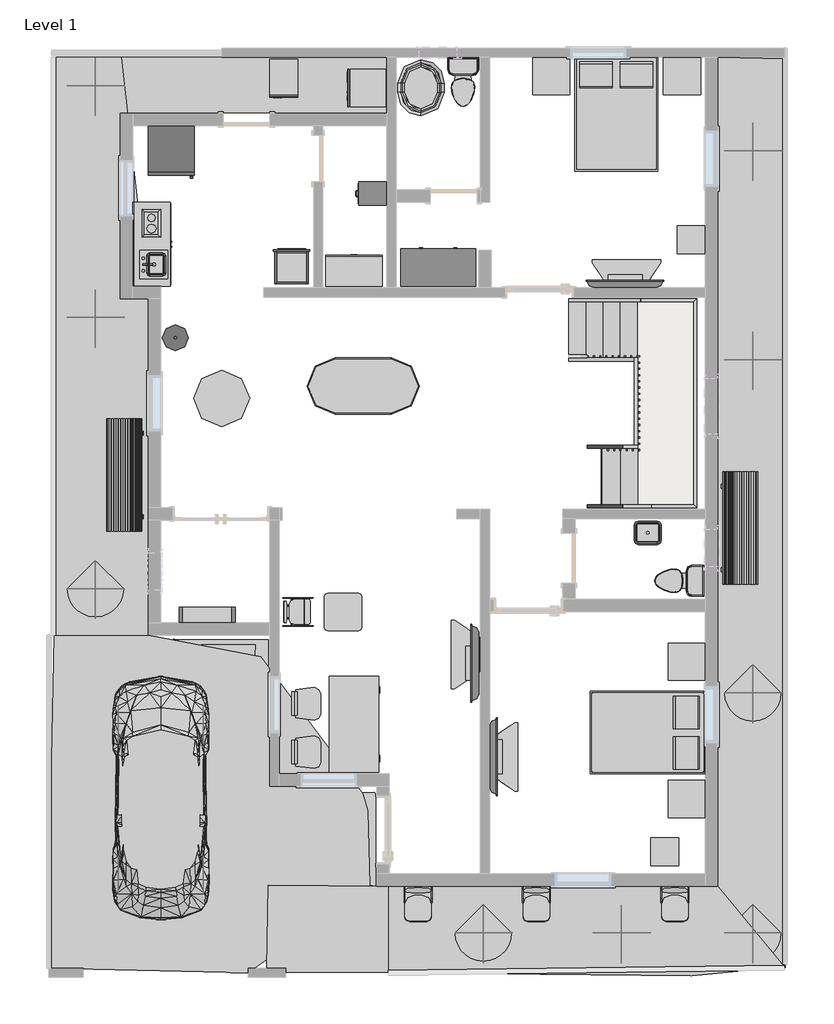
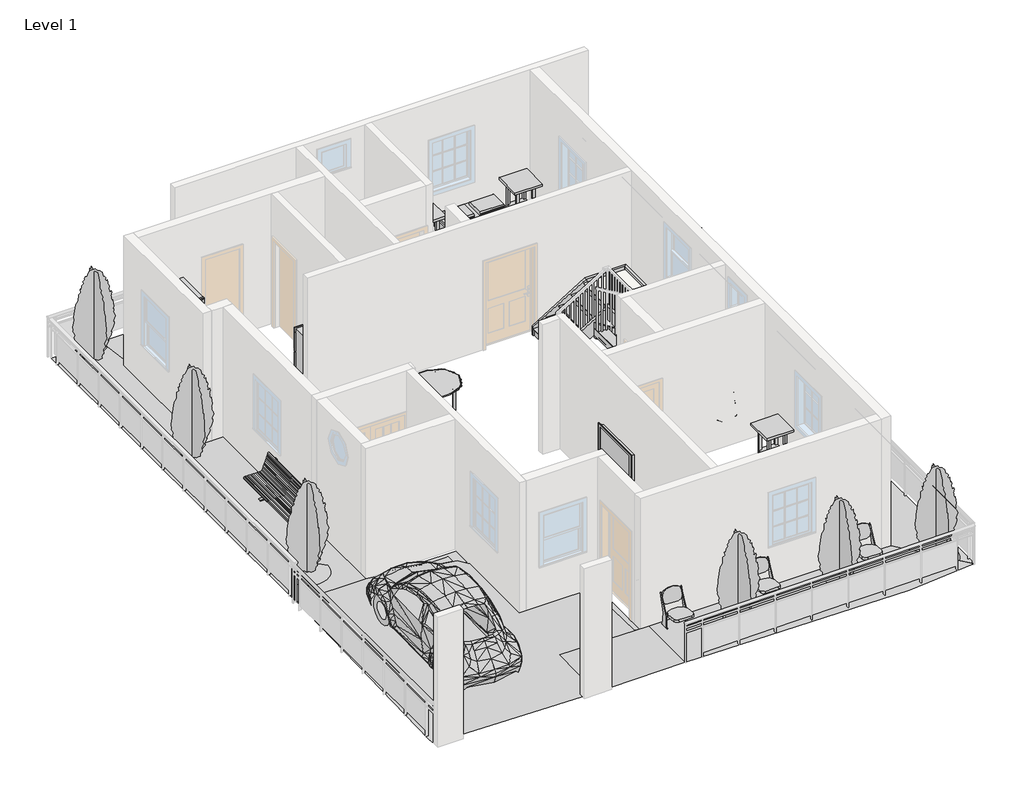
# One storey, part 4 of 4: 29 furniture elements, 16 proxies, 11 geographic elements, 8 members, 6 flow terminals, 2 stair flights, 1 slab.
"""IFC4 building model written with IfcOpenShell, lengths in millimetres."""

from ifc_helpers import new_model, si_unit, frame, origin, place, context, project, spatial, polyline, outline, extrude, faceted_brep, triangles, transform, mapped, element, save
from components import proxy_7e1014cc, proxy_fe84b772, proxy_45b28599, proxy_844211aa, proxy_8b8c2dc4, rpc_beetle_rpc_beetle_3ce7ba48, proxy_a13a33b2, flow_terminal_871c2e40, flow_terminal_d49f872f, flow_terminal_62a433f7, toilet_domestic_3d_toilet_domestic_3d_f7549cf7, toilet_domestic_3d_toilet_domestic_3d_183bbd19, flow_terminal_2ca5ee5d, furniture_c8abb964, furniture_b1353b55, chair_desk_chair_desk_ccc35c8f, chair_stacking_chair_stacking_4df0970f, furniture_95afb093, furniture_013ab306, furniture_9fa109b2, furniture_3d1d9cbc, furniture_417d203a, furniture_e1dba61b, furniture_fdf74506, tv_stand_tv_stand_6ce107e5, furniture_2c34a4f9, furniture_905aceb5, furniture_bcf351fa, furniture_097b63cf, furniture_5bc9ed15, geographic_element_235d1464, rpc_tree_conifer_chinese_juniper_7_1b9786cd, non_monolithic_landing_bdf883c6, stair_flight_1d7161dd, stair_flight_6800fc22

model = new_model("IFC4")

# Units and contexts
model_context = context("Model", 3, world=origin())
ifc_project = project(units=[si_unit("LENGTHUNIT", "METRE", prefix="MILLI")], contexts=[model_context])

# Site, building, storey
site = spatial("IfcSite", under=ifc_project)
building = spatial("IfcBuilding", under=site)
storey = spatial("IfcBuildingStorey", under=building, Name="Level 1", Elevation=0.0)

# Proxies
placement = place(None, origin())
element("IfcBuildingElementProxy", 1, Name="Building Element Proxy", at=placement, inside=storey, context=model_context, shape_type="Tessellation", body=[
    triangles([(-6292.1432602, 15373.2430298, 0.0), (-5213.9224457, 15356.2475555, 0.0), (-6292.1432602, 1860.4426907, 0.0), (-5190.4186478, 530.1176785, 0.0)], [[1, 3, 2], [4, 2, 3]], closed=False),
])
element("IfcBuildingElementProxy", 2, Name="Building Element Proxy", at=placement, inside=storey, context=model_context, shape_type="Tessellation", body=[
    triangles([(-6292.1432602, 1860.4426907, 0.0), (-5209.4686478, 549.1676785, 0.0), (-6721.6182083, 398.6723588, 0.0), (-11662.7439331, 449.442661, 0.0), (-11662.7439331, 1860.4426907, 0.0)], [[5, 4, 3], [3, 2, 1], [3, 1, 5]], closed=False),
])
element("IfcBuildingElementProxy", 3, Name="Building Element Proxy", at=placement, inside=storey, context=model_context, shape_type="Tessellation", body=[
    triangles([(-13339.1439331, 449.442661, 0.0), (-11669.2121429, 458.8875423, 0.0), (-11662.7439331, 1860.4426907, 0.0), (-13622.0394562, 1880.1632893, 0.0), (-13643.9439331, 525.642661, 0.0)], [[4, 5, 1], [1, 2, 3], [1, 3, 4]], closed=False),
])
element("IfcBuildingElementProxy", 4, Name="Building Element Proxy", at=placement, inside=storey, context=model_context, shape_type="Tessellation", body=[
    triangles([(-15577.8398438, 5952.1611053, 0.0), (-17123.743158, 5952.1611053, 0.0), (-15577.8398438, 11438.5611053, 0.0), (-16035.0398438, 11438.5611053, 0.0), (-16021.9080872, 15373.2430298, 0.0), (-17123.743158, 15373.2430298, 0.0)], [[6, 2, 4], [4, 2, 1], [6, 4, 5], [4, 3, 5], [3, 4, 1]], closed=False),
])
element("IfcBuildingElementProxy", 5, Name="Building Element Proxy", at=placement, inside=storey, context=model_context, shape_type="Tessellation", body=[
    triangles([(-16013.146994, 15373.2430298, 0.0), (-16019.2815033, 15373.2430298, 0.0), (-15917.9969879, 14469.5377258, 0.0), (-11691.6398438, 14461.1614929, 0.0), (-11691.6398438, 15373.2430298, 0.0)], [[3, 5, 1], [1, 2, 3], [3, 4, 5]], closed=False),
])
element("IfcBuildingElementProxy", 6, Name="Building Element Proxy", at=placement, inside=storey, context=model_context, shape_type="Tessellation", body=[
    triangles([(-17114.218158, 5945.8109116, 0.0), (-15577.8398438, 5952.1611053, 0.0), (-15719.3253937, 5575.8137283, 0.0), (-13765.4318665, 5526.4318588, 0.0), (-13747.9236328, 5599.4901901, 0.0), (-13732.6571228, 3093.6073906, 0.0), (-11998.7943512, 3091.0264435, 0.0), (-11972.09133, 1876.438662, 0.0), (-13622.0394562, 1891.7326412, 0.0), (-16641.1435455, 525.642661, 0.0), (-17217.7350952, 675.719874, 0.0), (-17199.943158, 525.642661, 0.0), (-13948.7439331, 449.442661, 0.0), (-12085.333255, 3366.7753098, 0.0)], [[12, 13, 10], [6, 11, 10], [12, 10, 11], [1, 11, 3], [3, 2, 1], [6, 3, 11], [3, 4, 2], [9, 10, 13], [9, 8, 7], [8, 9, 13], [9, 7, 6], [4, 5, 2], [5, 4, 14], [6, 14, 4], [14, 6, 7], [4, 3, 6], [9, 6, 10]], closed=False),
])
element("IfcBuildingElementProxy", 7, Name="Building Element Proxy", at=placement, inside=storey, context=model_context, shape_type="Tessellation", body=[
    triangles([(-13839.5657135, 5779.0495789, 0.0), (-13853.3788239, 5648.8115982, 0.0), (-14738.6096741, 5792.6731659, 0.0), (-13837.1100494, 5794.7480392, 0.0), (-13844.1212494, 5616.9437759, 0.0), (-14719.3480591, 5791.5819534, 0.0), (-14720.0968506, 5784.5259888, 0.0)], [[3, 7, 6], [6, 7, 2], [3, 6, 4], [2, 5, 1], [5, 2, 7], [1, 4, 6], [4, 1, 5], [2, 1, 6]], closed=False),
])
element("IfcBuildingElementProxy", 8, Name="Building Element Proxy", at=placement, inside=storey, context=model_context, shape_type="Tessellation", body=[
    triangles([(-11869.4394562, 3361.3611053, 0.0), (-11892.5240936, 3389.4227646, 0.0), (-12081.1823456, 3388.4777641, 0.0), (-11869.4394562, 1862.7610085, 0.0), (-11970.361203, 1873.1361019, 0.0), (-12092.2537628, 3386.2162743, 0.0)], [[3, 6, 1], [1, 6, 5], [3, 1, 2], [1, 5, 4]], closed=False),
])
element("IfcBuildingElementProxy", 9, Name="Building Element Proxy", at=placement, inside=storey, context=model_context, shape_type="Tessellation", body=[
    triangles([(-13622.0394562, 5455.0077301, 0.0), (-13622.0394562, 5882.7031357, 0.0), (-15168.4729706, 5887.4801697, 0.0)], [[3, 1, 2]], closed=False),
])
proxy_shape = proxy_7e1014cc(model_context)
element("IfcBuildingElementProxy", 10, Name="18\" x 24\" x 34 1/2\"", ObjectType="18\" x 24\" x 34 1/2\"", at=placement, inside=storey, context=model_context, shape_type="MappedRepresentation", body=[
    mapped(proxy_shape, transform((-13674.1574653, 14776.5930991, 0.0), x_axis=(1.0, 0.0, 0.0), y_axis=(0.0, 1.0, 0.0), z_axis=(0.0, 0.0, 1.0))),
])
proxy_2_shape = proxy_fe84b772(model_context)
element("IfcBuildingElementProxy", 11, Name="Cook Top-2 Unit : 12\" x 18\"", ObjectType="Cook Top-2 Unit : 12\" x 18\"", at=placement, inside=storey, context=model_context, shape_type="MappedRepresentation", body=[
    mapped(proxy_2_shape, transform((-15450.8399968, 12700.6858539, 0.0), x_axis=(-1.0, 0.0, 0.0), y_axis=(0.0, -1.0, 0.0), z_axis=(0.0, 0.0, 1.0))),
])
proxy_3_shape = proxy_45b28599(model_context)
element("IfcBuildingElementProxy", 12, Name="Dishwasher : 24\" x 24\" x 34\"", ObjectType="Dishwasher : 24\" x 24\" x 34\"", at=placement, inside=storey, context=model_context, shape_type="MappedRepresentation", body=[
    mapped(proxy_3_shape, transform((-12277.1574653, 15259.1930991, 0.0), x_axis=(0.0, -1.0000000000000007, 0.0), y_axis=(1.0000000000000007, 0.0, 0.0), z_axis=(0.0, 0.0, 1.0))),
])
proxy_4_shape = proxy_844211aa(model_context)
element("IfcBuildingElementProxy", 13, Name="Kitchenette - Small : 54\"", ObjectType="Kitchenette - Small : 54\"", at=placement, inside=storey, context=model_context, shape_type="MappedRepresentation", body=[
    mapped(proxy_4_shape, transform((-15831.8399968, 12308.8233534, 0.0), x_axis=(0.0, 1.0, 0.0), y_axis=(-1.0, 0.0, 0.0), z_axis=(0.0, 0.0, 1.0))),
])
proxy_5_shape = proxy_8b8c2dc4(model_context)
element("IfcBuildingElementProxy", 14, Name="Oven Double-Built-in : 21 1/2\" x 39 1/4\" x 21\"", ObjectType="Oven Double-Built-in : 21 1/2\" x 39 1/4\" x 21\"", at=placement, inside=storey, context=model_context, shape_type="MappedRepresentation", body=[
    mapped(proxy_5_shape, transform((-13276.2149241, 12087.6269172, 0.0), x_axis=(-1.0000000000000004, 0.0, 0.0), y_axis=(0.0, -1.0000000000000004, 0.0), z_axis=(0.0, 0.0, 1.0))),
])
rpc_beetle_rpc_beetle_shape = rpc_beetle_rpc_beetle_3ce7ba48(model_context)
element("IfcBuildingElementProxy", 15, Name="RPC Beetle : RPC Beetle", ObjectType="RPC Beetle : RPC Beetle", at=placement, inside=storey, context=model_context, shape_type="MappedRepresentation", body=[
    mapped(rpc_beetle_rpc_beetle_shape, transform((-15374.6399968, 2063.6426639, 0.0), x_axis=(1.0, 0.0, 0.0), y_axis=(0.0, 1.0, 0.0), z_axis=(0.0, 0.0, 1.0))),
])
proxy_6_shape = proxy_a13a33b2(model_context)
element("IfcBuildingElementProxy", 16, Name="Refrigerator : 30\" x 32\" RH", ObjectType="Refrigerator : 30\" x 32\" RH", at=placement, inside=storey, context=model_context, shape_type="MappedRepresentation", body=[
    mapped(proxy_6_shape, transform((-15204.7774968, 13869.4120868, 0.0), x_axis=(1.0, 0.0, 0.0), y_axis=(0.0, 1.0, 0.0), z_axis=(0.0, 0.0, 1.0))),
])

# Flow terminals
flow_terminal_shape = flow_terminal_871c2e40(model_context)
element("IfcFlowTerminal", 17, ObjectType="Sink Kitchen-Island : 18\" x 18\"", at=placement, inside=storey, context=model_context, shape_type="MappedRepresentation", body=[
    mapped(flow_terminal_shape, transform((-15486.5945957, 11981.6718177, 0.0), x_axis=(0.0, 1.0, 0.0), y_axis=(-1.0, 0.0, 0.0), z_axis=(0.0, 0.0, 1.0))),
])
flow_terminal_2_shape = flow_terminal_d49f872f(model_context)
element("IfcFlowTerminal", 18, ObjectType="Sink Vanity-Round : 19\" x 19\"", at=placement, inside=storey, context=model_context, shape_type="MappedRepresentation", body=[
    mapped(flow_terminal_2_shape, transform((-15053.3054094, 10706.9093177, 609.6), x_axis=(0.0, 1.0000000000000002, 0.0), y_axis=(-1.0000000000000002, 0.0, 0.0), z_axis=(0.0, 0.0, 1.0))),
])
flow_terminal_3_shape = flow_terminal_62a433f7(model_context)
element("IfcFlowTerminal", 19, ObjectType="Sink Vanity-Square : 20\" x 18\"", at=placement, inside=storey, context=model_context, shape_type="MappedRepresentation", body=[
    mapped(flow_terminal_3_shape, transform((-7450.8327199, 7674.6972628, 609.6), x_axis=(1.0, 0.0, 0.0), y_axis=(0.0, 1.0, 0.0), z_axis=(0.0, 0.0, 1.0))),
])
toilet_domestic_3d_toilet_domestic_3d_shape = toilet_domestic_3d_toilet_domestic_3d_f7549cf7(model_context)
toilet_domestic_3d_toilet_domestic_3d_2_shape = toilet_domestic_3d_toilet_domestic_3d_183bbd19(model_context)
element("IfcFlowTerminal", 20, ObjectType="Toilet-Domestic-3D : Toilet-Domestic-3D", at=placement, inside=storey, context=model_context, shape_type="MappedRepresentation", body=[
    mapped(toilet_domestic_3d_toilet_domestic_3d_shape, transform((-7015.4395067, 6841.1610583, 0.0), x_axis=(0.0, -1.0000000000000002, 0.0), y_axis=(1.0000000000000002, 0.0, 0.0), z_axis=(0.0, 0.0, 1.0))),
    mapped(toilet_domestic_3d_toilet_domestic_3d_2_shape, transform((-7015.4395067, 6841.1610583, 0.0), x_axis=(0.0, -1.0000000000000002, 0.0), y_axis=(1.0000000000000002, 0.0, 0.0), z_axis=(0.0, 0.0, 1.0))),
])
element("IfcFlowTerminal", 21, ObjectType="Toilet-Domestic-3D : Toilet-Domestic-3D", at=placement, inside=storey, context=model_context, shape_type="MappedRepresentation", body=[
    mapped(toilet_domestic_3d_toilet_domestic_3d_shape, transform((-10447.0399968, 14878.5466366, 0.0), x_axis=(1.0, 0.0, 0.0), y_axis=(0.0, 1.0, 0.0), z_axis=(0.0, 0.0, 1.0))),
    mapped(toilet_domestic_3d_toilet_domestic_3d_2_shape, transform((-10447.0399968, 14878.5466366, 0.0), x_axis=(1.0, 0.0, 0.0), y_axis=(0.0, 1.0, 0.0), z_axis=(0.0, 0.0, 1.0))),
])
flow_terminal_4_shape = flow_terminal_2ca5ee5d(model_context)
element("IfcFlowTerminal", 22, ObjectType="Tub-Free Standing-3D : 30\" x 60\"", at=placement, inside=storey, context=model_context, shape_type="MappedRepresentation", body=[
    mapped(flow_terminal_4_shape, transform((-11132.8399968, 14878.5466366, 0.0), x_axis=(1.0, 0.0, 0.0), y_axis=(0.0, 1.0, 0.0), z_axis=(0.0, 0.0, 1.0))),
])

# Furniture
furniture_shape = furniture_c8abb964(model_context)
element("IfcFurniture", 23, ObjectType="Bed-Box : Double 53\" x 74\"", at=placement, inside=storey, context=model_context, shape_type="MappedRepresentation", body=[
    mapped(furniture_shape, transform((-8288.0399968, 14695.5905665, 0.0), x_axis=(1.0, 0.0, 0.0), y_axis=(0.0, 1.0, 0.0), z_axis=(0.0, 0.0, 1.0))),
])
element("IfcFurniture", 24, ObjectType="Bed-Box : Double 53\" x 74\"", at=placement, inside=storey, context=model_context, shape_type="MappedRepresentation", body=[
    mapped(furniture_shape, transform((-7200.7139711, 4703.8135173, 0.0), x_axis=(0.0, -0.9999999999999999, 0.0), y_axis=(0.9999999999999999, 0.0, 0.0), z_axis=(0.0, 0.0, 1.0))),
])
furniture_2_shape = furniture_b1353b55(model_context)
element("IfcFurniture", 25, ObjectType="Cabinet-File 4 Drawer : 15\" x 18\"", at=placement, inside=storey, context=model_context, shape_type="MappedRepresentation", body=[
    mapped(furniture_2_shape, transform((-11778.1056967, 13025.1646112, 0.0), x_axis=(0.0, -0.9999999999999998, 0.0), y_axis=(0.9999999999999998, 0.0, 0.0), z_axis=(0.0, 0.0, 1.0))),
])
chair_desk_chair_desk_shape = chair_desk_chair_desk_ccc35c8f(model_context)
element("IfcFurniture", 26, ObjectType="Chair-Desk : Chair-Desk", at=placement, inside=storey, context=model_context, shape_type="MappedRepresentation", body=[
    mapped(chair_desk_chair_desk_shape, transform((-13175.5434793, 4047.1610583, 0.0), x_axis=(0.0, -1.0000000000000004, 0.0), y_axis=(1.0000000000000004, 0.0, 0.0), z_axis=(0.0, 0.0, 1.0))),
])
element("IfcFurniture", 27, ObjectType="Chair-Desk : Chair-Desk", at=placement, inside=storey, context=model_context, shape_type="MappedRepresentation", body=[
    mapped(chair_desk_chair_desk_shape, transform((-13175.5434793, 4834.5610583, 0.0), x_axis=(0.0, -1.0, 0.0), y_axis=(1.0, 0.0, 0.0), z_axis=(0.0, 0.0, 1.0))),
])
chair_stacking_chair_stacking_shape = chair_stacking_chair_stacking_4df0970f(model_context)
element("IfcFurniture", 28, ObjectType="Chair-Stacking : Chair-Stacking", at=placement, inside=storey, context=model_context, shape_type="MappedRepresentation", body=[
    mapped(chair_stacking_chair_stacking_shape, transform((-13248.3714604, 6154.1118779, 0.0), x_axis=(0.0, -1.0000000000000004, 0.0), y_axis=(1.0000000000000004, 0.0, 0.0), z_axis=(0.0, 0.0, 1.0))),
])
furniture_3_shape = furniture_95afb093(model_context)
element("IfcFurniture", 29, ObjectType="Counter Top w Sink Hole : 24\" Depth", at=placement, inside=storey, context=model_context, shape_type="MappedRepresentation", body=[
    mapped(furniture_3_shape, transform((-15831.8399968, 12842.2233534, 0.0), x_axis=(0.0, 1.0, 0.0), y_axis=(-1.0, 0.0, 0.0), z_axis=(0.0, 0.0, 1.0))),
])
furniture_4_shape = furniture_013ab306(model_context)
element("IfcFurniture", 30, ObjectType="Desk : 60\" x 30\" Student", at=placement, inside=storey, context=model_context, shape_type="MappedRepresentation", body=[
    mapped(furniture_4_shape, transform((-11844.0399968, 3740.0426639, 0.0), x_axis=(0.0, 1.0, 0.0), y_axis=(-1.0, 0.0, 0.0), z_axis=(0.0, 0.0, 1.0))),
])
furniture_5_shape = furniture_9fa109b2(model_context)
element("IfcFurniture", 31, ObjectType="Dresser : 48\" x 72\" x 24\"", at=placement, inside=storey, context=model_context, shape_type="MappedRepresentation", body=[
    mapped(furniture_5_shape, transform((-11122.6332566, 11583.3981042, 0.0), x_axis=(-1.0000000000000004, 0.0, 0.0), y_axis=(0.0, -1.0000000000000004, 0.0), z_axis=(0.0, 0.0, 1.0))),
])
furniture_6_shape = furniture_3d1d9cbc(model_context)
element("IfcFurniture", 32, ObjectType="Seating-Auditorium : 18\" x 24\" x 30\"", at=placement, inside=storey, context=model_context, shape_type="MappedRepresentation", body=[
    mapped(furniture_6_shape, transform((-11019.4156105, 1782.3180737, 0.0), x_axis=(-1.0000000000000002, 0.0, 0.0), y_axis=(0.0, -1.0000000000000002, 0.0), z_axis=(0.0, 0.0, 1.0))),
])
element("IfcFurniture", 33, ObjectType="Seating-Auditorium : 18\" x 24\" x 30\"", at=placement, inside=storey, context=model_context, shape_type="MappedRepresentation", body=[
    mapped(furniture_6_shape, transform((-9092.5121279, 1782.3180737, 0.0), x_axis=(-1.0, 0.0, 0.0), y_axis=(0.0, -1.0, 0.0), z_axis=(0.0, 0.0, 1.0))),
])
element("IfcFurniture", 34, ObjectType="Seating-Auditorium : 18\" x 24\" x 30\"", at=placement, inside=storey, context=model_context, shape_type="MappedRepresentation", body=[
    mapped(furniture_6_shape, transform((-6831.9121279, 1782.3180737, 0.0), x_axis=(-1.0, 0.0, 0.0), y_axis=(0.0, -1.0, 0.0), z_axis=(0.0, 0.0, 1.0))),
])
furniture_7_shape = furniture_417d203a(model_context)
element("IfcFurniture", 35, ObjectType="Shelving : 36\" x 10\" x 72\"", at=placement, inside=storey, context=model_context, shape_type="MappedRepresentation", body=[
    mapped(furniture_7_shape, transform((-14620.7704522, 6587.1610583, 0.0), x_axis=(1.0, 0.0, 0.0), y_axis=(0.0, 1.0, 0.0), z_axis=(0.0, 0.0, 1.0))),
])
furniture_8_shape = furniture_e1dba61b(model_context)
element("IfcFurniture", 36, ObjectType="Storage Pedestal : 20\" x 36\" x 36\"", at=placement, inside=storey, context=model_context, shape_type="MappedRepresentation", body=[
    mapped(furniture_8_shape, transform((-12405.0625107, 10961.4426822, 0.0), x_axis=(-1.0000000000000004, 0.0, 0.0), y_axis=(0.0, -1.0000000000000004, 0.0), z_axis=(0.0, 0.0, 1.0))),
])
furniture_9_shape = furniture_fdf74506(model_context)
element("IfcFurniture", 37, ObjectType="TV - Flat Screen : 50\"", at=placement, inside=storey, context=model_context, shape_type="MappedRepresentation", body=[
    mapped(furniture_9_shape, transform((-9956.7013731, 3974.9055724, 914.4), x_axis=(0.0, 1.0, 0.0), y_axis=(-1.0, 0.0, 0.0), z_axis=(0.0, 0.0, 1.0))),
])
element("IfcFurniture", 38, ObjectType="TV - Flat Screen : 50\"", at=placement, inside=storey, context=model_context, shape_type="MappedRepresentation", body=[
    mapped(furniture_9_shape, transform((-7809.3845109, 11674.8996819, 914.4), x_axis=(-1.0, 0.0, 0.0), y_axis=(0.0, -1.0, 0.0), z_axis=(0.0, 0.0, 1.0))),
])
element("IfcFurniture", 39, ObjectType="TV - Flat Screen : 50\"", at=placement, inside=storey, context=model_context, shape_type="MappedRepresentation", body=[
    mapped(furniture_9_shape, transform((-10251.5786204, 5491.0165441, 914.4), x_axis=(0.0, -1.0000000000000004, 0.0), y_axis=(1.0000000000000004, 0.0, 0.0), z_axis=(0.0, 0.0, 1.0))),
])
tv_stand_tv_stand_shape = tv_stand_tv_stand_6ce107e5(model_context)
element("IfcFurniture", 40, ObjectType="TV Stand : TV Stand", at=placement, inside=storey, context=model_context, shape_type="MappedRepresentation", body=[
    mapped(tv_stand_tv_stand_shape, transform((-7654.8519947, 11616.3610583, 0.0), x_axis=(-1.0000000000000004, 0.0, 0.0), y_axis=(0.0, -1.0000000000000004, 0.0), z_axis=(0.0, 0.0, 1.0))),
])
element("IfcFurniture", 41, ObjectType="TV Stand : TV Stand", at=placement, inside=storey, context=model_context, shape_type="MappedRepresentation", body=[
    mapped(tv_stand_tv_stand_shape, transform((-10015.2399968, 3845.7730562, 0.0), x_axis=(0.0, 1.0000000000000013, 0.0), y_axis=(-1.0000000000000013, 0.0, 0.0), z_axis=(0.0, 0.0, 1.0))),
])
element("IfcFurniture", 42, ObjectType="TV Stand : TV Stand", at=placement, inside=storey, context=model_context, shape_type="MappedRepresentation", body=[
    mapped(tv_stand_tv_stand_shape, transform((-10178.3434793, 5765.2737788, 0.0), x_axis=(0.0, -1.0000000000000007, 0.0), y_axis=(1.0000000000000007, 0.0, 0.0), z_axis=(0.0, 0.0, 1.0))),
])
furniture_10_shape = furniture_2c34a4f9(model_context)
element("IfcFurniture", 43, ObjectType="Table-Dining Oval : 36\" x 72\"", at=placement, inside=storey, context=model_context, shape_type="MappedRepresentation", body=[
    mapped(furniture_10_shape, transform((-11670.8203246, 10374.2594189, 0.0), x_axis=(1.0, 0.0, 0.0), y_axis=(0.0, 1.0, 0.0), z_axis=(0.0, 0.0, 1.0))),
])
furniture_11_shape = furniture_905aceb5(model_context)
element("IfcFurniture", 44, ObjectType="Table-Dining Round w Chairs : 36\" Diameter", at=placement, inside=storey, context=model_context, shape_type="MappedRepresentation", body=[
    mapped(furniture_11_shape, transform((-14487.721964, 9997.8397468, 0.0), x_axis=(1.0, 0.0, 0.0), y_axis=(0.0, 1.0, 0.0), z_axis=(0.0, 0.0, 1.0))),
])
furniture_12_shape = furniture_bcf351fa(model_context)
element("IfcFurniture", 45, ObjectType="Table-End : 24\" x 24\"", at=placement, inside=storey, context=model_context, shape_type="MappedRepresentation", body=[
    mapped(furniture_12_shape, transform((-12711.3736271, 6180.7610583, 0.0), x_axis=(1.0, 0.0, 0.0), y_axis=(0.0, 1.0, 0.0), z_axis=(0.0, 0.0, 1.0))),
])
furniture_13_shape = furniture_097b63cf(model_context)
element("IfcFurniture", 46, ObjectType="Table-Night Stand : 18\" x 18\" x 24\"", at=placement, inside=storey, context=model_context, shape_type="MappedRepresentation", body=[
    mapped(furniture_13_shape, transform((-7388.0771096, 2192.9610583, 0.0), x_axis=(1.0, 0.0, 0.0), y_axis=(0.0, 1.0, 0.0), z_axis=(0.0, 0.0, 1.0))),
])
element("IfcFurniture", 47, ObjectType="Table-Night Stand : 18\" x 18\" x 24\"", at=placement, inside=storey, context=model_context, shape_type="MappedRepresentation", body=[
    mapped(furniture_13_shape, transform((-6956.2771096, 12175.1610583, 0.0), x_axis=(1.0, 0.0, 0.0), y_axis=(0.0, 1.0, 0.0), z_axis=(0.0, 0.0, 1.0))),
])
furniture_14_shape = furniture_5bc9ed15(model_context)
element("IfcFurniture", 48, ObjectType="Table-Night Stand : 24\" x 24\" x 30\"", at=placement, inside=storey, context=model_context, shape_type="MappedRepresentation", body=[
    mapped(furniture_14_shape, transform((-7184.8771096, 14763.6426639, 0.0), x_axis=(1.0, 0.0, 0.0), y_axis=(0.0, 1.0, 0.0), z_axis=(0.0, 0.0, 1.0))),
])
element("IfcFurniture", 49, ObjectType="Table-Night Stand : 24\" x 24\" x 30\"", at=placement, inside=storey, context=model_context, shape_type="MappedRepresentation", body=[
    mapped(furniture_14_shape, transform((-9318.4771096, 14763.6426639, 0.0), x_axis=(1.0, 0.0, 0.0), y_axis=(0.0, 1.0, 0.0), z_axis=(0.0, 0.0, 1.0))),
])
element("IfcFurniture", 50, ObjectType="Table-Night Stand : 24\" x 24\" x 30\"", at=placement, inside=storey, context=model_context, shape_type="MappedRepresentation", body=[
    mapped(furniture_14_shape, transform((-7108.6771096, 5215.5610583, 0.0), x_axis=(1.0, 0.0, 0.0), y_axis=(0.0, 1.0, 0.0), z_axis=(0.0, 0.0, 1.0))),
])
element("IfcFurniture", 51, ObjectType="Table-Night Stand : 24\" x 24\" x 30\"", at=placement, inside=storey, context=model_context, shape_type="MappedRepresentation", body=[
    mapped(furniture_14_shape, transform((-7108.6771096, 2980.3610583, 0.0), x_axis=(1.0, 0.0, 0.0), y_axis=(0.0, 1.0, 0.0), z_axis=(0.0, 0.0, 1.0))),
])

# Geographic elements
geographic_element_shape = geographic_element_235d1464(model_context)
element("IfcGeographicElement", 52, ObjectType="Park Bench : 72\"", at=placement, inside=storey, context=model_context, shape_type="MappedRepresentation", body=[
    mapped(geographic_element_shape, transform((-5961.9434793, 7702.4426639, 0.0), x_axis=(0.0, 1.0000000000000002, 0.0), y_axis=(-1.0000000000000002, 0.0, 0.0), z_axis=(0.0, 0.0, 1.0))),
])
element("IfcGeographicElement", 53, ObjectType="Park Bench : 72\"", at=placement, inside=storey, context=model_context, shape_type="MappedRepresentation", body=[
    mapped(geographic_element_shape, transform((-15933.4399968, 8566.0426639, 0.0), x_axis=(0.0, -1.0000000000000002, 0.0), y_axis=(1.0000000000000002, 0.0, 0.0), z_axis=(0.0, 0.0, 1.0))),
])
rpc_tree_conifer_chinese_juniper_7_shape = rpc_tree_conifer_chinese_juniper_7_1b9786cd(model_context)
element("IfcGeographicElement", 54, ObjectType="RPC Tree - Conifer : Chinese Juniper - 7'", at=placement, inside=storey, context=model_context, shape_type="MappedRepresentation", body=[
    mapped(rpc_tree_conifer_chinese_juniper_7_shape, transform((-16441.6366679, 6711.8426639, 0.0), x_axis=(1.0, 0.0, 0.0), y_axis=(0.0, 1.0, 0.0), z_axis=(0.0, 0.0, 1.0))),
])
element("IfcGeographicElement", 55, ObjectType="RPC Tree - Conifer : Chinese Juniper - 7'", at=placement, inside=storey, context=model_context, shape_type="MappedRepresentation", body=[
    mapped(rpc_tree_conifer_chinese_juniper_7_shape, transform((-16441.6366679, 11133.7610583, 0.0), x_axis=(1.0, 0.0, 0.0), y_axis=(0.0, 1.0, 0.0), z_axis=(0.0, 0.0, 1.0))),
])
element("IfcGeographicElement", 56, ObjectType="RPC Tree - Conifer : Chinese Juniper - 7'", at=placement, inside=storey, context=model_context, shape_type="MappedRepresentation", body=[
    mapped(rpc_tree_conifer_chinese_juniper_7_shape, transform((-16441.6366679, 14916.0426639, 0.0), x_axis=(1.0, 0.0, 0.0), y_axis=(0.0, 1.0, 0.0), z_axis=(0.0, 0.0, 1.0))),
])
element("IfcGeographicElement", 57, ObjectType="RPC Tree - Conifer : Chinese Juniper - 7'", at=placement, inside=storey, context=model_context, shape_type="MappedRepresentation", body=[
    mapped(rpc_tree_conifer_chinese_juniper_7_shape, transform((-5722.8366679, 13851.5610583, 0.0), x_axis=(1.0, 0.0, 0.0), y_axis=(0.0, 1.0, 0.0), z_axis=(0.0, 0.0, 1.0))),
])
element("IfcGeographicElement", 58, ObjectType="RPC Tree - Conifer : Chinese Juniper - 7'", at=placement, inside=storey, context=model_context, shape_type="MappedRepresentation", body=[
    mapped(rpc_tree_conifer_chinese_juniper_7_shape, transform((-5722.8366679, 10447.9610583, 0.0), x_axis=(1.0, 0.0, 0.0), y_axis=(0.0, 1.0, 0.0), z_axis=(0.0, 0.0, 1.0))),
])
element("IfcGeographicElement", 59, ObjectType="RPC Tree - Conifer : Chinese Juniper - 7'", at=placement, inside=storey, context=model_context, shape_type="MappedRepresentation", body=[
    mapped(rpc_tree_conifer_chinese_juniper_7_shape, transform((-5722.8366679, 5012.3610583, 0.0), x_axis=(1.0, 0.0, 0.0), y_axis=(0.0, 1.0, 0.0), z_axis=(0.0, 0.0, 1.0))),
])
element("IfcGeographicElement", 60, ObjectType="RPC Tree - Conifer : Chinese Juniper - 7'", at=placement, inside=storey, context=model_context, shape_type="MappedRepresentation", body=[
    mapped(rpc_tree_conifer_chinese_juniper_7_shape, transform((-10117.0366679, 1098.4426639, 0.0), x_axis=(1.0, 0.0, 0.0), y_axis=(0.0, 1.0, 0.0), z_axis=(0.0, 0.0, 1.0))),
])
element("IfcGeographicElement", 61, ObjectType="RPC Tree - Conifer : Chinese Juniper - 7'", at=placement, inside=storey, context=model_context, shape_type="MappedRepresentation", body=[
    mapped(rpc_tree_conifer_chinese_juniper_7_shape, transform((-7867.1401504, 1098.4426639, 0.0), x_axis=(1.0, 0.0, 0.0), y_axis=(0.0, 1.0, 0.0), z_axis=(0.0, 0.0, 1.0))),
])
element("IfcGeographicElement", 62, ObjectType="RPC Tree - Conifer : Chinese Juniper - 7'", at=placement, inside=storey, context=model_context, shape_type="MappedRepresentation", body=[
    mapped(rpc_tree_conifer_chinese_juniper_7_shape, transform((-5722.8366679, 1098.4426639, 0.0), x_axis=(1.0, 0.0, 0.0), y_axis=(0.0, 1.0, 0.0), z_axis=(0.0, 0.0, 1.0))),
])

# Members
element("IfcMember", 63, ObjectType="Stringer - 2\" Width", at=placement, inside=storey, context=model_context, shape_type="SweptSolid", body=[
    extrude(outline(polyline([(212.114512, -8719.8399968), (0.0, -8719.8399968), (0.0, -8481.754485), (618.0666667, -7461.944485), (922.8666667, -7547.0989415), (212.114512, -8719.8399968)])), frame((0.0, 11387.7610583, 0.0), z_axis=(0.0, 1.0, 0.0), x_axis=(0.0, 0.0, 1.0)), (0.0, 0.0, 1.0), 50.8),
])
element("IfcMember", 64, ObjectType="Stringer - 2\" Width", at=placement, inside=storey, context=model_context, shape_type="SweptSolid", body=[
    extrude(outline(polyline([(212.114512, -8719.8399968), (0.0, -8719.8399968), (0.0, -8481.754485), (502.251205, -7653.0399968), (858.6599665, -7653.0399968), (212.114512, -8719.8399968)])), frame((0.0, 10422.5610583, 0.0), z_axis=(0.0, 1.0, 0.0), x_axis=(0.0, 0.0, 1.0)), (0.0, 0.0, 1.0), 50.8),
])
element("IfcMember", 65, ObjectType="Stringer - 2\" Width", at=placement, inside=storey, context=model_context, shape_type="SweptSolid", body=[
    extrude(outline(polyline([(618.0666667, -7463.1355086), (922.8666667, -7377.981052), (1736.114512, -8719.8399968), (1379.7057504, -8719.8399968), (618.0666667, -7463.1355086)])), frame((0.0, 8032.6426639, 0.0), z_axis=(0.0, 1.0, 0.0), x_axis=(0.0, 0.0, 1.0)), (0.0, 0.0, 1.0), 50.8),
])
element("IfcMember", 66, ObjectType="Stringer - 2\" Width", at=placement, inside=storey, context=model_context, shape_type="SweptSolid", body=[
    extrude(outline(polyline([(702.3724171, -7602.2399968), (1058.7811786, -7602.2399968), (1736.114512, -8719.8399968), (1379.7057504, -8719.8399968), (702.3724171, -7602.2399968)])), frame((0.0, 8997.8426639, 0.0), z_axis=(0.0, 1.0, 0.0), x_axis=(0.0, 0.0, 1.0)), (0.0, 0.0, 1.0), 50.8),
])
element("IfcMember", 67, ObjectType="Stringer - 2\" Width", at=placement, inside=storey, context=model_context, shape_type="Brep", body=[
    faceted_brep([(-7377.981052, 8083.4426639, 922.8666667), (-7377.981052, 8032.6426639, 922.8666667), (-6637.0399968, 8032.6426639, 922.8666667), (-6687.8399968, 8083.4426639, 922.8666667), (-7463.1355086, 8083.4426639, 618.0666667), (-6687.8399968, 8083.4426639, 618.0666667), (-7463.1355086, 8032.6426639, 618.0666667), (-6637.0399968, 8032.6426639, 618.0666667)], [[[0, 1, 2, 3]], [[4, 0, 3, 5]], [[6, 4, 5, 7]], [[1, 6, 7, 2]], [[1, 0, 4, 6]], [[2, 7, 5, 3]]]),
])
element("IfcMember", 68, ObjectType="Stringer - 2\" Width", at=placement, inside=storey, context=model_context, shape_type="SweptSolid", body=[
    extrude(outline(polyline([(-6637.0399968, 8032.6426639), (-6687.8399968, 8083.4426639), (-6687.8399968, 11387.7610583), (-6637.0399968, 11438.5610583), (-6637.0399968, 8032.6426639)])), frame((0.0, 0.0, 618.0666667), z_axis=(0.0, 0.0, 1.0), x_axis=(1.0, 0.0, 0.0)), (0.0, 0.0, 1.0), 304.8),
])
element("IfcMember", 69, ObjectType="Stringer - 2\" Width", at=placement, inside=storey, context=model_context, shape_type="Brep", body=[
    faceted_brep([(-6687.8399968, 11387.7610583, 922.8666667), (-6637.0399968, 11438.5610583, 922.8666667), (-7547.0989415, 11438.5610583, 922.8666667), (-7547.0989415, 11387.7610583, 922.8666667), (-6687.8399968, 11387.7610583, 618.0666667), (-7461.944485, 11387.7610583, 618.0666667), (-6637.0399968, 11438.5610583, 618.0666667), (-7461.944485, 11438.5610583, 618.0666667)], [[[0, 1, 2, 3]], [[4, 0, 3, 5]], [[6, 4, 5, 7]], [[1, 6, 7, 2]], [[1, 0, 4, 6]], [[2, 7, 5, 3]]]),
])
element("IfcMember", 70, ObjectType="Stringer - 2\" Width", at=placement, inside=storey, context=model_context, shape_type="SweptSolid", body=[
    extrude(outline(polyline([(-7653.0399968, 10473.3610583), (-7602.2399968, 10473.3610583), (-7602.2399968, 9048.6426639), (-7653.0399968, 9048.6426639), (-7653.0399968, 10473.3610583)])), frame((0.0, 0.0, 618.0666667), z_axis=(0.0, 0.0, 1.0), x_axis=(1.0, 0.0, 0.0)), (0.0, 0.0, 1.0), 304.8),
])

# Slab
non_monolithic_landing_shape = non_monolithic_landing_bdf883c6(model_context)
element("IfcSlab", 71, ObjectType="Non-Monolithic Landing", at=placement, inside=storey, context=model_context, shape_type="MappedRepresentation", body=[
    mapped(non_monolithic_landing_shape, transform((0.0, 0.0, 0.0), x_axis=(1.0, 0.0, 0.0), y_axis=(0.0, 1.0, 0.0), z_axis=(0.0, 0.0, 1.0))),
])

# Stair flights
stair_flight_shape = stair_flight_1d7161dd(model_context)
element("IfcStairFlight", 72, ObjectType="2\" Tread 1\" Nosing 1/4\" Riser", at=placement, inside=storey, context=model_context, shape_type="MappedRepresentation", body=[
    mapped(stair_flight_shape, transform((0.0, 0.0, 0.0), x_axis=(1.0, 0.0, 0.0), y_axis=(0.0, 1.0, 0.0), z_axis=(0.0, 0.0, 1.0))),
])
stair_flight_2_shape = stair_flight_6800fc22(model_context)
element("IfcStairFlight", 73, ObjectType="2\" Tread 1\" Nosing 1/4\" Riser", at=placement, inside=storey, context=model_context, shape_type="MappedRepresentation", body=[
    mapped(stair_flight_2_shape, transform((0.0, 0.0, 0.0), x_axis=(1.0, 0.0, 0.0), y_axis=(0.0, 1.0, 0.0), z_axis=(0.0, 0.0, 1.0))),
])

save(model, "model.ifc")

# Revit data of these elements
# Type "18\" x 24\" x 34 1/2\""
#   Label = "T"
#   Assembly Code = "E1090400"
#   Depth = 2' - 0"
#   Height = 2' - 10 1/2"
#   Width = 1' - 6"
#   Panel Face Material = Plastic, Opaque Black
#   Trach Compact. Material = Steel, Paint Finish, Ivory, Matte
#   Default Elevation = 0
# Type "Cook Top-2 Unit : 12\" x 18\""
#   Assembly Code = "E1090400"
#   Counter Height = 3' - 0"
#   Depth = 1' - 6"
#   Width = 1' - 0"
#   Burner Material = Steel, Chrome Plated
#   Cooktop Material = Steel, Polished
#   Default Elevation = 0
# Type "Dishwasher : 24\" x 24\" x 34\""
#   Label = "DW"
#   Assembly Code = "E1090400"
#   Depth = 2' - 0"
#   Height = 2' - 10"
#   Width = 2' - 0"
#   Dishwasher Material = Steel, Paint Finish, Ivory, Glossy
#   Panel Face Material = Plastic, Opaque Black
#   Default Elevation = 0
# Type "Kitchenette - Small : 54\""
#   Assembly Code = "E1090400"
#   Width = 4' - 6"
#   Height = 2' - 10 1/2"
#   Depth = 2' - 0"
#   Toe Depth = 0' - 3"
#   Toe Height = 0' - 3 1/2"
#   Cabinet Material = Cabinets
#   Door/Drawer Material = Cabinets
#   Handle Material = Cabinets - Handles
#   Default Elevation = 0
# Type "Oven Double-Built-in : 21 1/2\" x 39 1/4\" x 21\""
#   Label = "OVEN"
#   Assembly Code = "E1090400"
#   Depth = 1' - 9"
#   Height = 3' - 3 1/4"
#   Width = 1' - 9 1/2"
#   Oven Material = Metal - Stainless Steel, Polished
#   Default Elevation = 0
# Type "RPC Beetle : RPC Beetle"
#   built-in parameter 1005195 = "RPC-16-0U6E-L4EG-ENH1-J3KF-SVEL-0TX4-C0"
#   Height = 0
# Type "Refrigerator : 30\" x 32\" RH"
#   Label = "REF."
#   Assembly Code = "E1090400"
#   Depth = 2' - 7 3/4"
#   Handle = 2' - 3"
#   Height = 5' - 10"
#   Rear Clearance = 0' - 2"
#   Top Door Height = 1' - 8"
#   Width = 2' - 5 3/8"
#   Material = Steel, Paint Finish, Ivory, Glossy
#   Default Elevation = 0
# Type "Sink Kitchen-Island : 18\" x 18\""
#   Assembly Code = "D2010410"
#   Counter Height = 3' - 0"
#   Depth = 1' - 6"
#   Width = 1' - 6"
#   Faucet Material = Steel, Polished
#   Sink Material = Steel, Polished
#   Default Elevation = 0
# Type "Sink Vanity-Round : 19\" x 19\""
#   Assembly Code = "D2010400"
#   Top Of Counter = 2' - 7"
#   Basin Material = Porcelain, Linen
#   Faucet Material = Steel, Polished
#   Default Elevation = 0
# Type "Sink Vanity-Square : 20\" x 18\""
#   Assembly Code = "D2010400"
#   Counter Height = 2' - 7"
#   Depth = 1' - 6"
#   Width = 1' - 8"
#   Basin Material = Porcelain, Linen
#   Faucet Material = Steel, Polished
#   Default Elevation = 0
# Type "Toilet-Domestic-3D : Toilet-Domestic-3D"
#   Assembly Code = "D2010110"
#   Toilet - Bowl/Basin Material = Porcelain, Linen
#   Toilet - Seat Material = Laminate, Linen, Matte
#   Default Elevation = 0
# Type "Tub-Free Standing-3D : 30\" x 60\""
#   Assembly Code = "D2010110"
#   Height = 1' - 6"
#   Length = 3' - 0"
#   Width = 2' - 6"
#   Tub Material = Porcelain, Ivory
#   Default Elevation = 0
# Type "Bed-Box : Double 53\" x 74\""
#   Assembly Code = "E2020200"
#   Length = 6' - 2"
#   Width = 4' - 5"
#   Frame Material = Birch
#   Mattress Material = Linen, White
#   Default Elevation = 0
# Type "Cabinet-File 4 Drawer : 15\" x 18\""
#   Assembly Code = "E2020200"
#   Depth = 1' - 6"
#   Height = 4' - 4"
#   Width = 1' - 3"
#   Cabinet Material = Steel, Paint Finish, Ivory, Glossy
#   Handle Material = Steel, Chrome Plated
#   Default Elevation = 0
# Type "Chair-Desk : Chair-Desk"
#   Assembly Code = "E2020200"
#   Seat/Back Material = Textile - Slate Blue
#   Base Material = Steel, Chrome Plated
#   Default Elevation = 0
# Type "Chair-Stacking : Chair-Stacking"
#   Assembly Code = "E2020200"
#   Seat/Back Material = Cherry
#   Default Elevation = 0
# Type "Counter Top w Sink Hole : 24\" Depth"
#   Assembly Code = "C1030400"
#   Counter Thickness = 0' - 1 1/2"
#   Depth [instance default] = 2' - 1"
#   Height = 3' - 0"
#   Length [instance default] = 8' - 0"
#   Sink Location [instance default] = 2' - 0"
#   Sink Location To Wall [instance default] = 0' - 6"
#   Sink Opening Depth [instance default] = 1' - 3"
#   Sink Opening Width [instance default] = 2' - 3"
#   Counter Top Material = none
#   Default Elevation = 0
# Type "Desk : 60\" x 30\" Student"
#   Assembly Code = "E2020200"
#   Depth = 2' - 6"
#   Height = 2' - 6"
#   Leg Height = 0' - 6"
#   Width = 5' - 0"
#   Body Material = Laminate, Ivory, Matte
#   Handle/Leg Material = Steel, Chrome Plated
#   Top Material = Cherry
#   Default Elevation = 0
# Type "Dresser : 48\" x 72\" x 24\""
#   Assembly Code = "E2020200"
#   Depth = 2' - 0"
#   Height = 6' - 0"
#   Width = 4' - 0"
#   Dresser Material = Laminate - Ivory, Glossy
#   Drawer Material = Laminate, Ivory, Matte
#   Knob Material = Cherry
#   Default Elevation = 0
# Type "Seating-Auditorium : 18\" x 24\" x 30\""
#   Assembly Code = "E2020200"
#   Seat Material = Linen, Beige
#   Frame Material = Steel, Paint Finish, Dark Gray, Matte
#   Default Elevation = 0
# Type "Shelving : 36\" x 10\" x 72\""
#   Assembly Code = "E2020200"
#   Depth = 0' - 10"
#   Height = 6' - 0"
#   Width = 3' - 0"
#   Shelving Unit Material = Birch
#   Default Elevation = 0
# Type "Storage Pedestal : 20\" x 36\" x 36\""
#   Assembly Code = "E2020"
#   Depth = 1' - 8"
#   Height = 3' - 0"
#   Width = 3' - 0"
#   Cabinet Material = Steel, Paint Finish, Ivory, Glossy
#   Handles Material = Steel, Chrome Plated
#   Default Elevation = 0
# Type "TV - Flat Screen : 50\""
#   SinAng = 0' - 0.0193"
#   L = 3' - 7.57782"
#   H = 2' - 0.51477"
#   Thickness = 0' - 4.33071"
#   Diagonal = 4' - 2"
#   CosAng = 0' - 0.03431"
#   Stand [instance default] = yes
#   Default Elevation = 0
# Type "TV Stand : TV Stand"
#   Depth = 1' - 6"
#   Width = 3' - 8"
#   Height = 1' - 7 1/2"
#   Finish = Melamine - Gray
#   Default Elevation = 0
# Type "Table-Dining Oval : 36\" x 72\""
#   Assembly Code = "E2020200"
#   Length = 6' - 0"
#   Width = 3' - 0"
#   Base Material = Steel, Chrome Plated
#   Top Material = Glass - Clear, Grey
#   Default Elevation = 0
#   Description = (empty or 0)
# Type "Table-Dining Round w Chairs : 36\" Diameter"
#   Assembly Code = "E2020200"
#   Radius = 1' - 6"
#   Diameter = 3' - 0"
#   Height = 2' - 6"
#   Chairs = 4
#   Base Material = Pine
#   Top Material = Laminate, Linen, Matte
#   Default Elevation = 0
# Type "Table-End : 24\" x 24\""
#   Assembly Code = "E2020200"
#   Height = 2' - 6"
#   Length = 2' - 0"
#   Width = 2' - 0"
#   Base Material = Birch
#   Top Material = Laminate, Ivory, Matte
#   Default Elevation = 0
# Type "Table-Night Stand : 18\" x 18\" x 24\""
#   Assembly Code = "E2020200"
#   Depth = 1' - 6"
#   Height = 2' - 0"
#   Width = 1' - 6"
#   Base Material = Birch
#   Top Material = Laminate, Ivory, Matte
#   Default Elevation = 0
# Type "Table-Night Stand : 24\" x 24\" x 30\""
#   Assembly Code = "E2020200"
#   Depth = 2' - 0"
#   Height = 2' - 6"
#   Width = 2' - 0"
#   Base Material = Birch
#   Top Material = Laminate, Ivory, Matte
#   Default Elevation = 0
# Type "Park Bench : 72\""
#   Length = 6' - 0"
#   Seat Material = Wood - Teak
#   Frame Material = Steel, Paint Finish, Dark Gray, Matte
# Type "RPC Tree - Conifer : Chinese Juniper - 7'"
#   built-in parameter 1005198 = "{2, 15},{39, RPC-16-FUM3-UUQ0-UBF0-N000-ST1L-LVER-AU},{1, 0},{1, 0},{2, 13},{1, 8},{5, Color},{1, 0},{1, 0},{3, 0.8},{3, 0.8},{3, 0.8},{1, 8},{7, BBoxMin},{1, 0},{1, 0},{1, 0},{1, 0},{1, 0},{1, 8},{7, BBoxMax},{1, 0},{1, 0},{1, 0},{1, 0},{1, 0},{2, 11},{9, RPCTypeId},{1, 0},{1, 0},{39, RPC-16-FUM3-UUQ0-UBF0-N000-ST1L-LVER-AU},{1, 6},{14, RPCPlantHeight},{1, 0},{1, 0},{1, 7},{2, 11},{7, keyword},{1, 0},{1, 0},{34, :RPCs:Trees [General]:Geometry:RPC},{2, 11},{8, category},{1, 0},{1, 0},{15, Trees [General]},{2, 11},{12, LocalizedUID},{1, 0},{1, 0},{15, Chinese Juniper},{2, 14},{6, Height},{1, 0},{1, 0},{1, 7},{1, 2},{16, Cast Reflections},{1, 0},{1, 0},{1, 0},{1, 2},{12, Cast Shadows},{1, 0},{1, 0},{1, 1},{1, 2},{9, Lock View},{1, 0},{1, 0},{1, 0},{1, 4},{5, ViewC},{1, 0},{1, 0},{1, 0},{21, assetlibrary_base.fbx},{1, 5},"
#   built-in parameter 1005195 = "RPC-16-FUM3-UUQ0-UBF0-N000-ST1L-LVER-AU"
#   Type Comments = "Chinese Juniper"
#   Assembly Code = "G2050500"
#   Height = 7' - 0"
#   Description = (empty or 0)
#   Default Elevation = 0
# Elements 1, 2, 3, 4 (IfcBuildingElementProxy)
#   Material = Default Mass Zone
#   Phase Created = New Construction
# Elements 5, 6, 7, 8, 9 (IfcBuildingElementProxy)
#   Material = none
#   Phase Created = New Construction
# Element 10 (IfcBuildingElementProxy, "18\" x 24\" x 34 1/2\"")
#   Phase Created = New Construction
#   Materials on its faces: "Steel, Paint Finish, Ivory, Matte", "Plastic, Opaque Black"
# Element 11 (IfcBuildingElementProxy, "Cook Top-2 Unit : 12\" x 18\"")
#   Phase Created = New Construction
#   Materials on its faces: "Steel, Chrome Plated", "Steel, Polished"
# Element 12 (IfcBuildingElementProxy, "Dishwasher : 24\" x 24\" x 34\"")
#   Phase Created = New Construction
#   Materials on its faces: "Steel, Paint Finish, Ivory, Glossy", "Plastic, Opaque Black"
# Element 13 (IfcBuildingElementProxy, "Kitchenette - Small : 54\"")
#   Phase Created = New Construction
#   Materials on its faces: "Cabinets", "Cabinets - Handles"
# Element 14 (IfcBuildingElementProxy, "Oven Double-Built-in : 21 1/2\" x 39 1/4\" x 21\"")
#   Phase Created = New Construction
#   Materials on its faces: "Steel", "Metal - Stainless Steel, Polished", "Glass"
# Element 15 (IfcBuildingElementProxy, "RPC Beetle : RPC Beetle")
#   Phase Created = New Construction
# Element 16 (IfcBuildingElementProxy, "Refrigerator : 30\" x 32\" RH")
#   Phase Created = New Construction
#   Materials on its faces: "Steel, Paint Finish, Ivory, Glossy", "Steel, Chrome Plated"
# Element 17 (IfcFlowTerminal, "Sink Kitchen-Island : 18\" x 18\"")
#   Mark = "8"
#   Phase Created = New Construction
#   Materials on its faces: "Steel, Polished"
# Element 18 (IfcFlowTerminal, "Sink Vanity-Round : 19\" x 19\"")
#   Mark = "9"
#   Phase Created = New Construction
#   Materials on its faces: "Porcelain, Linen", "Steel, Polished"
# Element 19 (IfcFlowTerminal, "Sink Vanity-Square : 20\" x 18\"")
#   Mark = "4"
#   Phase Created = New Construction
#   Materials on its faces: "Porcelain, Linen", "Steel, Polished"
# Element 20 (IfcFlowTerminal, "Toilet-Domestic-3D : Toilet-Domestic-3D")
#   Mark = "1"
#   Phase Created = New Construction
#   Materials on its faces: "Porcelain, Linen", "Laminate, Linen, Matte"
# Element 21 (IfcFlowTerminal, "Toilet-Domestic-3D : Toilet-Domestic-3D")
#   Mark = "6"
#   Phase Created = New Construction
#   Materials on its faces: "Porcelain, Linen", "Laminate, Linen, Matte"
# Element 22 (IfcFlowTerminal, "Tub-Free Standing-3D : 30\" x 60\"")
#   Mark = "7"
#   Phase Created = New Construction
#   Materials on its faces: "Porcelain, Ivory"
# Elements 23, 24 (IfcFurniture, "Bed-Box : Double 53\" x 74\"")
#   Phase Created = New Construction
#   Materials on its faces: "Birch", "Linen, White"
# Element 25 (IfcFurniture, "Cabinet-File 4 Drawer : 15\" x 18\"")
#   Phase Created = New Construction
#   Materials on its faces: "Steel, Chrome Plated", "Steel, Paint Finish, Ivory, Glossy"
# Elements 26, 27 (IfcFurniture, "Chair-Desk : Chair-Desk")
#   Phase Created = New Construction
#   Materials on its faces: "Steel, Chrome Plated", "Textile - Slate Blue"
# Element 28 (IfcFurniture, "Chair-Stacking : Chair-Stacking")
#   Phase Created = New Construction
#   Materials on its faces: "Steel, Chrome Plated", "Cherry"
# Element 29 (IfcFurniture, "Counter Top w Sink Hole : 24\" Depth")
#   Sink Opening Depth = 1' - 3"
#   Sink Location To Wall = 0' - 6"
#   Length = 4' - 6"
#   Sink Location = 1' - 2"
#   Sink Opening Width = 1' - 4"
#   Depth = 2' - 0"
#   Phase Created = New Construction
#   Materials on its faces: "Counter Top"
# Element 30 (IfcFurniture, "Desk : 60\" x 30\" Student")
#   Phase Created = New Construction
#   Materials on its faces: "Steel, Chrome Plated", "Laminate, Ivory, Matte", "Cherry"
# Element 31 (IfcFurniture, "Dresser : 48\" x 72\" x 24\"")
#   Phase Created = New Construction
#   Materials on its faces: "Laminate, Ivory, Matte", "Cherry", "Laminate - Ivory, Glossy"
# Elements 32, 33, 34 (IfcFurniture, "Seating-Auditorium : 18\" x 24\" x 30\"")
#   Phase Created = New Construction
#   Materials on its faces: "Steel, Paint Finish, Dark Gray, Matte", "Linen, Beige"
# Element 35 (IfcFurniture, "Shelving : 36\" x 10\" x 72\"")
#   Phase Created = New Construction
#   Materials on its faces: "Birch"
# Element 36 (IfcFurniture, "Storage Pedestal : 20\" x 36\" x 36\"")
#   Phase Created = New Construction
#   Materials on its faces: "Steel, Paint Finish, Ivory, Glossy", "Steel, Chrome Plated"
# Elements 37, 38, 39 (IfcFurniture, "TV - Flat Screen : 50\"")
#   Stand = yes
#   Phase Created = New Construction
#   Materials on its faces: "TV - Black", "TV - Glass", "TV - Screen"
# Elements 40, 41, 42 (IfcFurniture, "TV Stand : TV Stand")
#   Phase Created = New Construction
#   Materials on its faces: "Melamine - Gray", "Glass - Shelves"
# Element 43 (IfcFurniture, "Table-Dining Oval : 36\" x 72\"")
#   Phase Created = New Construction
#   Materials on its faces: "Steel, Chrome Plated", "Glass - Clear, Grey"
# Element 44 (IfcFurniture, "Table-Dining Round w Chairs : 36\" Diameter")
#   Phase Created = New Construction
#   Materials on its faces: "Pine", "Laminate, Linen, Matte"
# Element 45 (IfcFurniture, "Table-End : 24\" x 24\"")
#   Phase Created = New Construction
#   Materials on its faces: "Laminate, Ivory, Matte", "Birch"
# Elements 46, 47 (IfcFurniture, "Table-Night Stand : 18\" x 18\" x 24\"")
#   Phase Created = New Construction
#   Materials on its faces: "Birch", "Laminate, Ivory, Matte"
# Elements 48, 49, 50, 51 (IfcFurniture, "Table-Night Stand : 24\" x 24\" x 30\"")
#   Phase Created = New Construction
#   Materials on its faces: "Birch", "Laminate, Ivory, Matte"
# Elements 52, 53 (IfcGeographicElement, "Park Bench : 72\"")
#   Phase Created = New Construction
#   Materials on its faces: "Wood - Teak", "Steel, Paint Finish, Dark Gray, Matte"
# Elements 54, 55, 56, 57, 58, 59, 60, 61, 62 (IfcGeographicElement, "RPC Tree - Conifer : Chinese Juniper - 7'")
#   Phase Created = New Construction
# Elements 63, 64, 65, 66, 67, 68, 69, 70 (IfcMember, "Stringer - 2\" Width")
#   Phase Created = New Construction
# Element 71 (IfcSlab, "Non-Monolithic Landing")
#   Phase Created = New Construction
# Elements 72, 73 (IfcStairFlight, "2\" Tread 1\" Nosing 1/4\" Riser")
#   Phase Created = New Construction
# Materials
#   "Plastic, Opaque Black": class "Plastic", colour RGB 0 0 0, transparency 0.7, Description = "Plastic, generic, opaque black", Cost = 0
#   "Steel, Paint Finish, Ivory, Matte": class "Metal", colour RGB 247 247 239, transparency 0, Description = "Steel, paint finish, ivory, matte", Cost = 0
#   "Steel, Chrome Plated": class "Metal", colour RGB 17 17 17, transparency 0, Description = "Chromiuim plated steel", Cost = 0
#   "Steel, Polished": class "Metal", colour RGB 57 57 57, transparency 0, Description = "Polished steel", Cost = 0
#   "Steel, Paint Finish, Ivory, Glossy": class "Metal", colour RGB 247 247 239, transparency 0, Description = "Steel, paint finish, ivory, glossy", Cost = 0
#   "Cabinets": colour RGB 249 249 249, transparency 0
#   "Cabinets - Handles": class "Metal", colour RGB 57 57 57, transparency 0
#   "Metal - Stainless Steel, Polished": class "Metal", colour RGB 216 216 216, transparency 0
#   "Porcelain, Linen": class "Ceramic", colour RGB 249 239 230, transparency 0, Description = "Porcelain, linen", Cost = 0
#   "Laminate, Linen, Matte": class "Plastic", colour RGB 249 239 230, transparency 0, Description = "Plastic Laminate - Linen, Matte", Cost = 0
#   "Porcelain, Ivory": class "Ceramic", colour RGB 247 247 239, transparency 0, Description = "Porcelain, ivory", Cost = 0
#   "Birch": class "Wood", colour RGB 224 178 126, transparency 0, Description = "Betula Alleghaniensis", Cost = 0
#   "Linen, White": class "Textile", colour RGB 247 247 239, transparency 0, Description = "Linen, white", Cost = 0
#   "Textile - Slate Blue": class "Fabric", colour RGB 98 102 118, transparency 0
#   "Cherry": class "Wood", colour RGB 226 177 128, transparency 0, Description = "Prunus Serotina", Cost = 0
#   "Laminate, Ivory, Matte": class "Plastic", colour RGB 247 247 239, transparency 0, Description = "Plastic Laminate - Ivory, Matte", Cost = 0
#   "Laminate - Ivory, Glossy": colour RGB 247 247 239, transparency 0
#   "Linen, Beige": class "Textile", colour RGB 249 239 230, transparency 0, Description = "Linen, beige", Cost = 0
#   "Steel, Paint Finish, Dark Gray, Matte": class "Metal", colour RGB 0 0 0, transparency 0, Description = "Steel, paint finish, dark gray, matte", Cost = 0
#   "Melamine - Gray": class "Wood", colour RGB 49 49 49, transparency 0
#   "Glass - Clear, Grey": class "Glass", colour RGB 252 255 255, transparency 0.64
#   "Pine": class "Wood", colour RGB 223 192 134, transparency 0, Description = "Pinus Echinata", Cost = 0
#   "Wood - Teak": class "Wood", colour RGB 120 73 19, transparency 0
#   "Default Mass Zone": class "Generic", colour RGB 0 255 0, transparency 0.5, Cost = 0
#   "Steel": class "Metal", colour RGB 247 247 247, transparency 0, Description = "Steel, mill finish", Cost = 0
#   "Glass": class "Glass", colour RGB 0 128 192, transparency 0.75, Description = "Soda Lime Glass", Cost = 0
#   "Counter Top": class "Wood", colour RGB 226 177 128, transparency 0
#   "TV - Black": colour RGB 49 49 49, transparency 0
#   "TV - Glass": colour RGB 157 157 157, transparency 0.9
#   "TV - Screen": colour RGB 0 0 0, transparency 0
#   "Glass - Shelves": class "Glass", colour RGB 167 167 167, transparency 0.9
